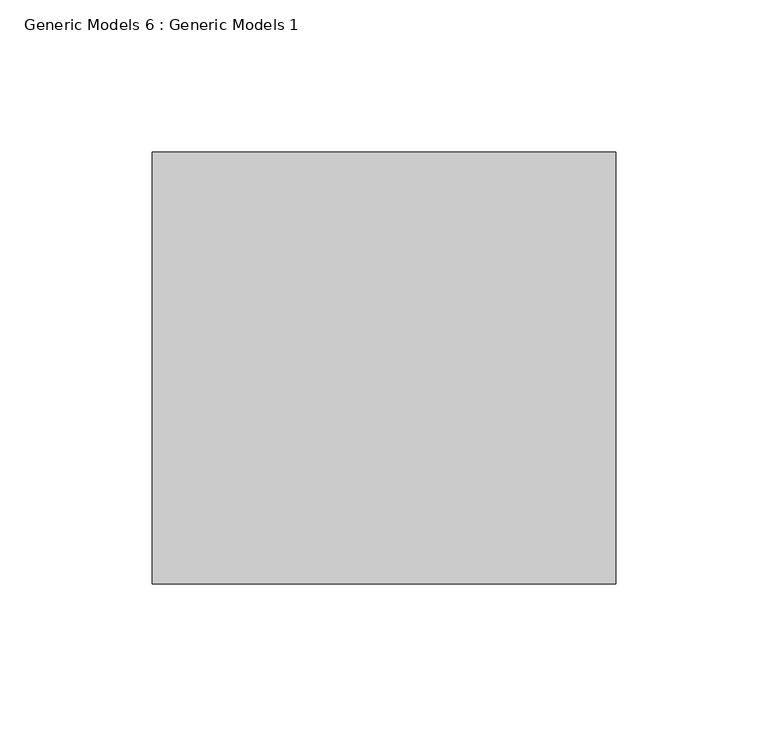
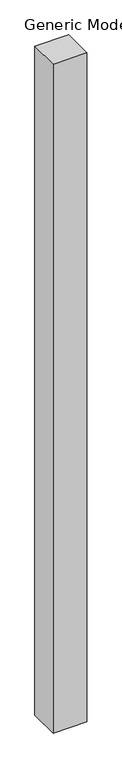
"""IFC4 building model written with IfcOpenShell, lengths in millimetres: proxy geometry, Generic Models 6 : Generic Models 1."""

from ifc_helpers import new_model, si_unit, origin, origin_with_axes, place, context, project, spatial, polyline, outline, extrude, source, transform, mapped, element, save


def generic_models_6_generic_models_1_d5b3bf35(model_context):
    return source(origin(), model_context, "Body", "SweptSolid", [
        extrude(outline(polyline([(-11070.9010638, -5471.7273102), (-10918.5010638, -5471.7273102), (-10918.5010638, -5613.7098142), (-11070.9010638, -5613.7098142), (-11070.9010638, -5471.7273102)])), origin_with_axes(), (0.0, 0.0, 1.0), 3200.4),
    ])


if __name__ == "__main__":
    model = new_model("IFC4")
    model_context = context("Model", 3, world=origin())
    ifc_project = project(units=[si_unit("LENGTHUNIT", "METRE", prefix="MILLI")], contexts=[model_context])
    site = spatial("IfcSite", under=ifc_project)
    building = spatial("IfcBuilding", under=site)
    placement = place(None, origin())
    generic_models_6_generic_models_1_shape = generic_models_6_generic_models_1_d5b3bf35(model_context)
    element("IfcBuildingElementProxy", 1, Name="Generic Models 6 : Generic Models 1", ObjectType="Generic Models 6 : Generic Models 1", at=placement, inside=building, context=model_context, shape_type="MappedRepresentation", body=[
        mapped(generic_models_6_generic_models_1_shape, transform((0.0, 0.0, 0.0), x_axis=(1.0, 0.0, 0.0), y_axis=(0.0, 1.0, 0.0), z_axis=(0.0, 0.0, 1.0))),
    ])
    save(model, "model.ifc")
